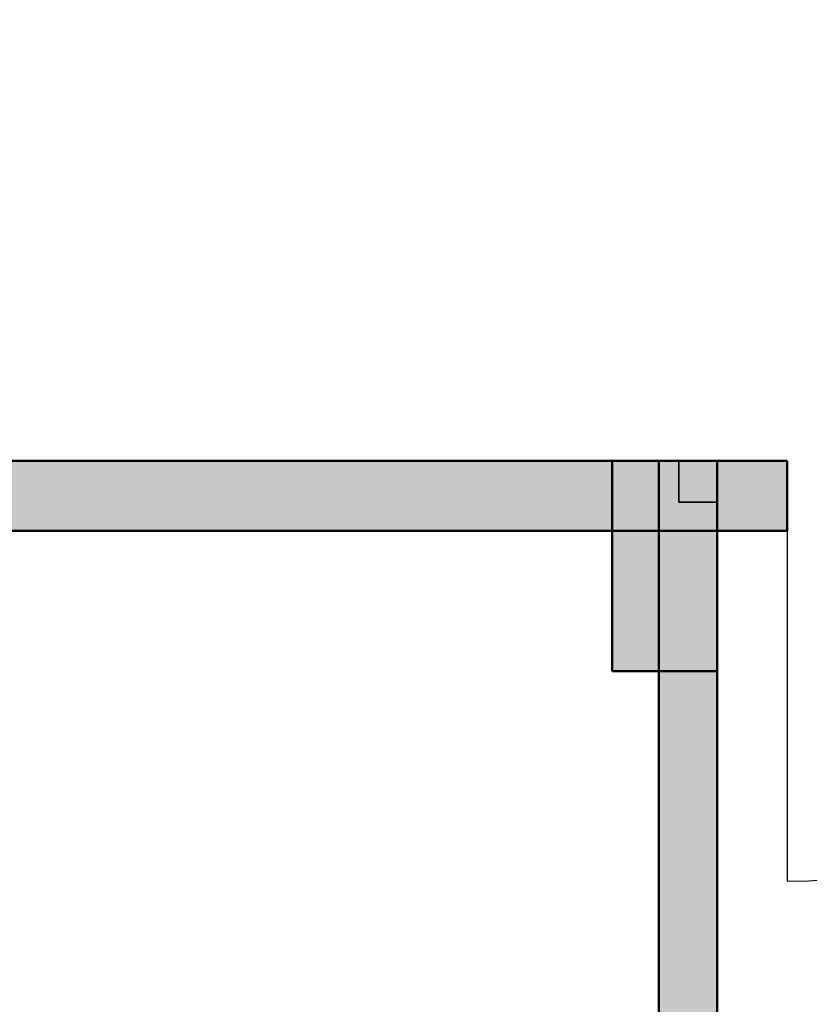
# Model space of a CAD drawing. Units: inches. Extents: x -7 to 1228, y -146 to 1091.
# Tile 33 of 88: x 747 to 815, y 446 to 531. Entities that reach past the tile are written whole.
import ezdxf

# ---------------------------------------------------------------- set-up
doc = ezdxf.new("R2010")
doc.units = ezdxf.units.IN
for name, color, linetype, lineweight in [('A-COLS', 6, 'Continuous', 35), ('A-DOOR', 4, 'Continuous', 25), ('A-WALL', 7, 'Continuous', 50), ('A-WALL-PATT', 251, 'Continuous', 13)]:
    doc.layers.add(name, color=color, linetype=linetype, lineweight=lineweight)

# ---------------------------------------------------------------- blocks, each defined once
blk = doc.blocks.new('DOOR-900')
blk.add_line((36, 0), (36, 36))
blk.add_arc((36, 0), 36, 90, 180)

msp = doc.modelspace()

# ---------------------------------------------------------------- hatches: boundary and pattern name
at = {"layer": 'A-COLS'}
h = msp.add_hatch(color=256, dxfattribs=at)
h.dxf.hatch_style = 1
h.paths.add_polyline_path([(807, 489.454), (803.711, 489.454), (803.711, 493), (798, 493), (798, 475), (807, 475)])
h = msp.add_hatch(color=256, dxfattribs=at)
h.dxf.hatch_style = 1
h.paths.add_polyline_path([(807, 489.454), (807, 493), (803.711, 493), (803.711, 489.454)])
at = {"layer": 'A-WALL-PATT'}
h = msp.add_hatch(color=256, dxfattribs=at)
h.dxf.hatch_style = 1
h.paths.add_polyline_path([(69, 568), (60, 568), (60, 493), (63.289, 493), (69, 493)])
h.paths.add_polyline_path([(69, 662.405), (60, 662.405), (60, 586), (69, 586)], flags=17)
h.paths.add_polyline_path([(69, 723), (184, 723), (184, 734), (179, 734), (179, 728), (69, 728), (69, 741.623), (60, 741.623), (60, 698.405), (69, 698.405)], flags=17)
h.paths.add_polyline_path([(69, 782), (231, 782), (231, 728), (231, 723), (231, 586), (236, 586), (236, 787), (69, 787), (69, 800.126), (60, 800.126), (60, 765.623), (69, 765.623)])
h.paths.add_polyline_path([(184, 842), (189, 842), (189, 848), (173, 848), (173, 842), (179, 842), (179, 787), (184, 787)])
h.paths.add_polyline_path([(118.22, 69), (69, 69), (69, 60), (118.22, 60)])
h.paths.add_polyline_path([(227, 69), (154.22, 69), (154.22, 60), (227, 60)])
h.paths.add_polyline_path([(236, 60), (232.711, 60), (227, 60), (227, 36), (236, 36)])
h.paths.add_polyline_path([(389, 60), (380, 60), (380, 36), (389, 36)])
h.paths.add_polyline_path([(384, 181), (380, 181), (380, 115), (380, 78), (384, 78)])
h.paths.add_polyline_path([(380, 115), (334.547, 115), (334.547, 109), (380, 109)])
h.paths.add_polyline_path([(274.547, 115), (236, 115), (236, 201), (232.711, 201), (231, 201), (231, 78), (236, 78), (236, 109), (274.547, 109)])
h.paths.add_polyline_path([(69, 123), (60, 123), (60, 78), (69, 78)])
h.paths.add_polyline_path([(69, 201), (60, 201), (60, 159), (69, 159)])
h.paths.add_polyline_path([(143, 219), (69, 219), (69, 213), (143, 213)], flags=17)
h.paths.add_polyline_path([(189, 219), (184, 219), (184, 274), (231, 274), (231, 219), (236, 219), (236, 279), (184, 279), (184, 297), (179, 297), (179, 279), (69, 279), (69, 290.912), (60, 290.912), (60, 262.179), (69, 262.179), (69, 274), (179, 274), (179, 219), (173, 219), (173, 213), (189, 213)])
h.paths.add_polyline_path([(69, 238.179), (60, 238.179), (60, 219), (69, 219)], flags=17)
h.paths.add_polyline_path([(69, 333), (60, 333), (60, 314.912), (69, 314.912), (69, 316.965)])
h.paths.add_polyline_path([(190, 338), (184, 338), (69, 338), (69, 333), (179, 333), (179, 327), (184, 327), (184, 333.021), (190, 333.046)])
h.paths.add_polyline_path([(69, 386.806), (60, 386.806), (60, 351), (69, 351)])
h.paths.add_polyline_path([(69, 475), (60, 475), (60, 422.806), (69, 422.806)])
h.paths.add_polyline_path([(236, 475), (231, 475), (231, 351.238), (236, 351.238)])
h.paths.add_polyline_path([(384, 475), (380, 475), (380, 362), (384, 362)])
h.paths.add_polyline_path([(547, 307), (439, 307), (439, 356), (445, 356), (445, 362), (433, 362), (433, 307), (380, 307), (380, 244), (380, 241), (384, 241), (384, 301), (433, 301), (433, 277), (439, 277), (439, 301), (547, 301)])
h.paths.add_polyline_path([(547, 241), (439, 241), (439, 247), (433, 247), (433, 235), (547, 235)])
h.paths.add_polyline_path([(450, 69), (440.286, 69), (424.889, 69), (389, 69), (389, 60), (450, 60)])
h.paths.add_polyline_path([(547, 69), (486, 69), (486, 60), (547, 60)])
h.paths.add_polyline_path([(556, 148.268), (547, 148.268), (547, 78), (556, 78)])
h.paths.add_polyline_path([(556, 223), (547, 223), (547, 195), (547, 184.268), (556, 184.268)])
h.paths.add_polyline_path([(556, 311.192), (547, 311.192), (547, 273.075), (556, 273.075)])
h.paths.add_polyline_path([(556, 344), (552.711, 344), (547, 344), (547, 335.192), (556, 335.192)])
h.paths.add_polyline_path([(556, 249.075), (547, 249.075), (547, 241), (556, 241)])
h.paths.add_polyline_path([(547, 362), (475, 362), (475, 356), (547, 356)], flags=0)
h.paths.add_polyline_path([(556, 399.621), (547, 399.621), (547, 362), (556, 362)])
h.paths.add_polyline_path([(556, 475), (547, 475), (547, 435.621), (556, 435.621)])
h.paths.add_polyline_path([(547, 493), (389, 493), (389, 487), (547, 487)])
h.paths.add_polyline_path([(380, 493), (278, 493), (278, 487), (380, 487)])
h.paths.add_polyline_path([(227, 493), (69, 493), (69, 487), (227, 487)])
h.paths.add_polyline_path([(643, 122.445), (634, 122.445), (634, 78), (643, 78)])
h.paths.add_polyline_path([(702.5, 69), (692.786, 69), (677.389, 69), (643, 69), (643, 60), (702.5, 60)])
h.paths.add_polyline_path([(798, 69), (738.5, 69), (738.5, 60), (798, 60)])
h.paths.add_polyline_path([(807, 60), (803.711, 60), (798, 60), (798, 36), (807, 36)])
h.paths.add_polyline_path([(807, 109), (846.751, 109), (846.751, 115), (807, 115), (807, 159), (802, 159), (802, 78), (807, 78)])
h.paths.add_polyline_path([(807, 201), (802, 201), (802, 195), (807, 195)])
h.paths.add_polyline_path([(643, 201), (634, 201), (634, 158.445), (643, 158.445)])
h.paths.add_polyline_path([(756, 225), (751, 225), (751, 219), (643, 219), (643, 213), (756, 213)])
h.paths.add_polyline_path([(643, 240.848), (634, 240.848), (634, 219), (643, 219)])
h.paths.add_polyline_path([(643, 274), (643, 288.629), (634, 288.629), (634, 264.848), (643, 264.848)])
h.paths.add_polyline_path([(802, 279), (756, 279), (756, 297), (751, 297), (751, 279), (643, 279), (643, 274), (751, 274), (751, 255), (756, 255), (756, 274), (802, 274)])
h.paths.add_polyline_path([(807, 333), (803.711, 333), (802, 333), (802, 279), (802, 274), (802, 219), (807, 219)])
h.paths.add_polyline_path([(956, 182), (951, 182), (951, 115), (906.751, 115), (906.751, 109), (951, 109), (951, 78), (956, 78)])
h.paths.add_polyline_path([(960, 60), (951, 60), (951, 36), (960, 36)])
h.paths.add_polyline_path([(1021, 69), (1005.781, 69), (960, 69), (960, 60), (1021, 60)])
h.paths.add_polyline_path([(956, 224), (951, 224), (951, 218), (956, 218)])
h.paths.add_polyline_path([(956, 302), (1004, 302), (1004, 278), (1010, 278), (1010, 302), (1118, 302), (1118, 290.809), (1127, 290.809), (1127, 326.968), (1118, 326.968), (1118, 320.966), (1118, 307), (1010, 307), (1010, 356), (1016, 356), (1016, 362), (1004, 362), (1004, 307), (951, 307), (951, 244), (951, 242), (954.289, 242), (956, 242)])
h.paths.add_polyline_path([(643, 333), (634, 333), (634, 312.629), (643, 312.629), (643, 316.965)])
h.paths.add_polyline_path([(756, 338), (643, 338), (643, 333), (751, 333), (751, 327), (756, 327)])
h.paths.add_polyline_path([(643, 388), (634, 388), (634, 351), (643, 351)])
h.paths.add_polyline_path([(807, 357), (802, 357), (802, 351), (807, 351)])
h.paths.add_polyline_path([(807, 475), (802, 475), (802, 393), (807, 393)])
h.paths.add_polyline_path([(643, 475), (634, 475), (634, 424), (643, 424)])
h.paths.add_polyline_path([(798, 493), (643, 493), (643, 487), (798, 487)])
h.paths.add_polyline_path([(634, 493), (556, 493), (556, 487), (634, 487)])
h.paths.add_polyline_path([(813, 493), (807, 493), (807, 487), (813, 487)])
h.paths.add_polyline_path([(951, 493), (849, 493), (849, 487), (951, 487)])
h.paths.add_polyline_path([(956, 484), (951, 484), (951, 374), (956, 374)])
h.paths.add_polyline_path([(1109, 493), (969, 493), (969, 487), (1109, 487)])
h.paths.add_polyline_path([(1127, 484), (1118, 484), (1118, 450.641), (1127, 450.641)])
h.paths.add_polyline_path([(1127, 414.641), (1118, 414.641), (1118, 365), (1127, 365)])
h.paths.add_polyline_path([(1109, 362), (1046, 362), (1046, 356), (1109, 356)], flags=17)
h.paths.add_polyline_path([(1127, 356), (1123.454, 356), (1118, 356), (1118, 350.968), (1127, 350.968)], flags=0)
h.paths.add_polyline_path([(1127, 266.809), (1118, 266.809), (1118, 262.361), (1118, 242), (1127, 242)], flags=17)
h.paths.add_polyline_path([(1118, 242), (1010, 242), (1010, 248), (1004, 248), (1004, 237), (1118, 237)])
h.paths.add_polyline_path([(1127, 224), (1118, 224), (1118, 170), (1127, 170)])
h.paths.add_polyline_path([(1127, 134), (1118, 134), (1118, 78), (1127, 78)])
h.paths.add_polyline_path([(1118, 69), (1057, 69), (1057, 60), (1118, 60)])
h.paths.add_polyline_path([(227, 571.546), (227, 574), (69, 574), (69, 568), (227, 568)])
h.paths.add_polyline_path([(380, 571.546), (380, 574), (278, 574), (278, 568), (380, 568)])
h.paths.add_polyline_path([(242, 574), (236, 574), (236, 568), (242, 568)])
h.paths.add_polyline_path([(547, 571.546), (547, 574), (389, 574), (389, 568), (547, 568)])
h.paths.add_polyline_path([(384, 733), (380, 733), (380, 586), (384, 586)])
h.paths.add_polyline_path([(556, 646), (634, 646), (634, 655), (547, 655), (547, 586), (556, 586)])
h.paths.add_polyline_path([(634, 574), (556, 574), (556, 568), (634, 568)])
h.paths.add_polyline_path([(643, 655), (634, 655), (634, 586), (643, 586)])
h.paths.add_polyline_path([(798, 574), (643, 574), (643, 568), (798, 568)])
h.paths.add_polyline_path([(643, 663.854), (634, 663.854), (634, 655), (643, 655)])
h.paths.add_polyline_path([(556, 676.967), (547, 676.967), (547, 655), (556, 655)])
h.paths.add_polyline_path([(556, 733), (547, 733), (547, 712.967), (556, 712.967)])
h.paths.add_polyline_path([(643, 710), (634, 710), (634, 699.854), (643, 699.854)])
h.paths.add_polyline_path([(807, 668), (802, 668), (802, 586), (807, 586)])
h.paths.add_polyline_path([(951, 574), (849, 574), (849, 568), (951, 568)])
h.paths.add_polyline_path([(956, 691), (951, 691), (951, 577), (956, 577)])
h.paths.add_polyline_path([(1109, 574), (969, 574), (969, 568), (1109, 568)])
h.paths.add_polyline_path([(1127, 643.403), (1118, 643.403), (1118, 577), (1127, 577)])
h.paths.add_polyline_path([(1127, 568), (1123.454, 568), (1118, 568), (1118, 493), (1127, 493)])
h.paths.add_polyline_path([(1127, 733), (1118, 733), (1118, 679.403), (1127, 679.403)])
h.paths.add_polyline_path([(1127, 777.348), (1118, 777.348), (1118, 770.035), (1118, 751), (1127, 751)], flags=17)
h.paths.add_polyline_path([(1118, 751), (1010, 751), (1010, 757), (1004, 757), (1004, 745), (1118, 745)])
h.paths.add_polyline_path([(956, 811), (1004, 811), (1004, 787), (1010, 787), (1010, 811), (1017.874, 811), (1017.874, 811.627, -0.414214), (1018.247, 812), (1031.978, 812, -0.414214), (1032.351, 811.627), (1032.351, 811), (1118, 811), (1118, 801.348), (1127, 801.348), (1127, 834.685), (1118, 834.685), (1118, 830.238), (1118, 817), (1010, 817), (1010, 866), (1016, 866), (1016, 872), (1004, 872), (1004, 817), (956, 817), (956, 866), (951, 866), (951, 751), (954.289, 751), (956, 751)])
h.paths.add_polyline_path([(1118, 872), (1046, 872), (1046, 866), (1118, 866)], flags=17)
h.paths.add_polyline_path([(1127, 924.711), (1118, 924.711), (1118, 884), (1127, 884)])
h.paths.add_polyline_path([(1127, 866), (1123.711, 866), (1118, 866), (1118, 858.685), (1127, 858.685)], flags=17)
h.paths.add_polyline_path([(956, 983), (951, 983), (951, 952), (807, 952), (807, 983), (802, 983), (802, 902), (807, 902), (807, 946), (951, 946), (951, 884), (956, 884)])
h.paths.add_polyline_path([(807, 842), (802, 842), (802, 787), (756, 787), (756, 806), (751, 806), (751, 787), (643, 787), (643, 782), (751, 782), (751, 764), (756, 764), (756, 782), (802, 782), (802, 728), (807, 728)])
h.paths.add_polyline_path([(756, 848), (643, 848), (643, 842), (751, 842), (751, 836), (756, 836)])
h.paths.add_polyline_path([(756, 734), (751, 734), (751, 728), (643, 728), (643, 723), (756, 723)])
h.paths.add_polyline_path([(643, 749.791), (634, 749.791), (634, 728), (637.289, 728), (643, 728)])
h.paths.add_polyline_path([(643, 805.405), (634, 805.405), (634, 773.791), (643, 773.791)])
h.paths.add_polyline_path([(643, 896.663), (634, 896.663), (634, 860), (637.289, 860), (643, 860)])
h.paths.add_polyline_path([(643, 842), (634, 842), (634, 829.405), (643, 829.405)])
h.paths.add_polyline_path([(643, 983), (634, 983), (634, 932.663), (643, 932.663)])
h.paths.add_polyline_path([(1127, 983), (1118, 983), (1118, 960.711), (1127, 960.711)])
h.paths.add_polyline_path([(1118, 1001), (1077.525, 1001), (1077.525, 992), (1118, 992)])
h.paths.add_polyline_path([(1041.525, 1001), (960, 1001), (960, 992), (1041.525, 992)])
h.paths.add_polyline_path([(960, 1025), (951, 1025), (951, 1001), (954.289, 1001), (960, 1001)])
h.paths.add_polyline_path([(807, 1025), (798, 1025), (798, 1001), (807, 1001)])
h.paths.add_polyline_path([(798, 1001), (738.5, 1001), (738.5, 992), (798, 992)])
h.paths.add_polyline_path([(702.5, 1001), (643, 1001), (643, 992), (702.5, 992)])
h.paths.add_polyline_path([(547, 1001), (499.113, 1001), (499.113, 992), (547, 992)])
h.paths.add_polyline_path([(463.113, 1001), (389, 1001), (389, 992), (463.113, 992)])
h.paths.add_polyline_path([(389, 1025), (380, 1025), (380, 1022), (380, 1001), (383.289, 1001), (389, 1001)])
h.paths.add_polyline_path([(236, 1025), (227, 1025), (227, 1001), (236, 1001)])
h.paths.add_polyline_path([(236, 983), (231, 983), (231, 860), (236, 860)])
h.paths.add_polyline_path([(274.547, 952), (236, 952), (236, 946), (274.547, 946)])
h.paths.add_polyline_path([(380, 952), (334.547, 952), (334.547, 946), (380, 946)])
h.paths.add_polyline_path([(384, 983), (380, 983), (380, 884), (383.289, 884), (384, 884)])
h.paths.add_polyline_path([(227, 1001), (155.012, 1001), (155.012, 992), (162.875, 992), (227, 992)])
h.paths.add_polyline_path([(119.012, 1001), (69, 1001), (69, 992), (119.012, 992)])
h.paths.add_polyline_path([(69, 983), (60, 983), (60, 922.987), (69, 922.987)])
h.paths.add_polyline_path([(69, 886.987), (60, 886.987), (60, 860), (63.289, 860), (69, 860)])
h.paths.add_polyline_path([(143, 848), (69, 848), (69, 842), (143, 842)])

# ---------------------------------------------------------------- linework, layer by layer
at = {"layer": 'A-COLS'}
msp.add_lwpolyline([(807, 493), (803.711, 493), (803.711, 489.454), (807, 489.454)], close=True, dxfattribs=at)
at = {"layer": 'A-WALL'}
for p, q in [((813, 493), (556, 493)), ((807, 493), (798, 493)), ((798, 493), (798, 475)), ((802, 393), (802, 493)), ((802, 493), (802, 392.651)), ((807, 393), (807, 493)), ((807, 475), (807, 493)), ((807, 493), (807, 487)), ((807, 493), (807, 393)), ((813, 493), (813, 487)), ((813, 487), (556, 487)), ((798, 475), (807, 475))]:
    msp.add_line(p, q, dxfattribs=at)

# ---------------------------------------------------------------- block references
at = {"layer": 'A-DOOR', "rotation": 180}
msp.add_blockref('DOOR-900', (849, 493), dxfattribs=at)

doc.saveas('drawing.dxf')
